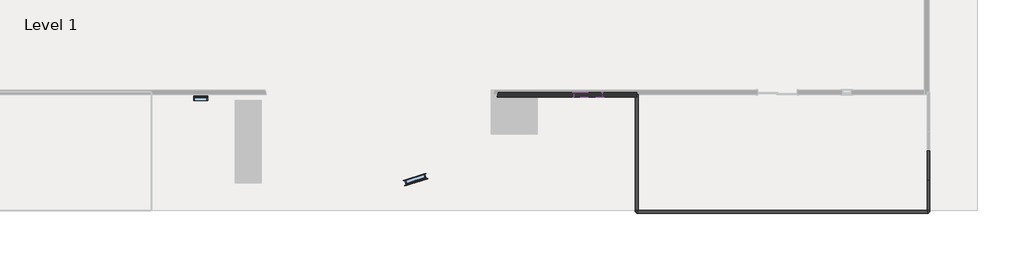
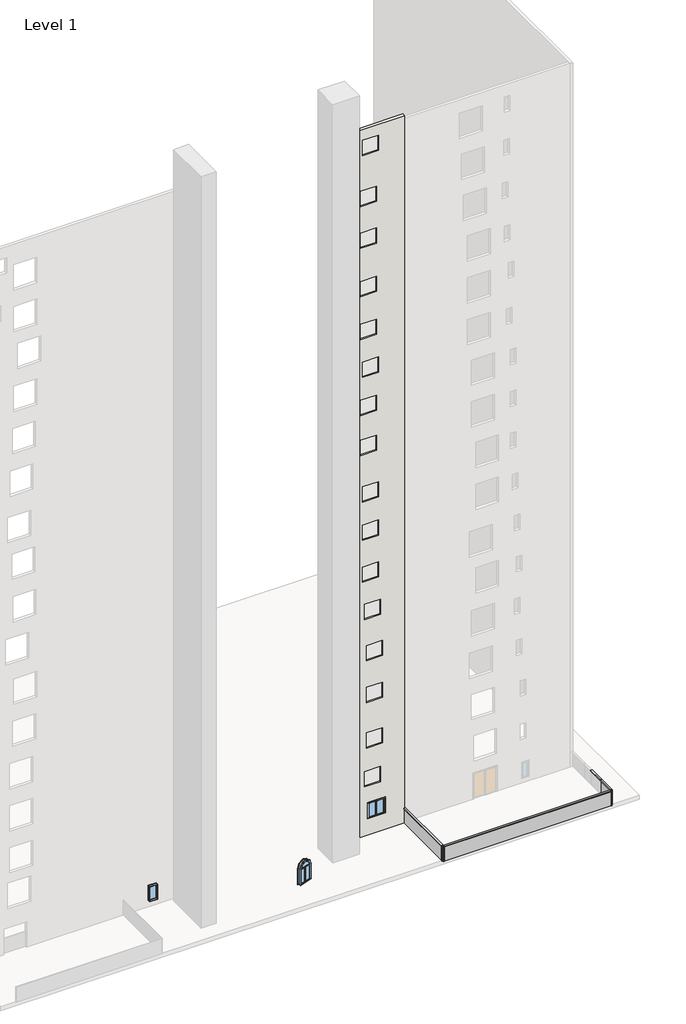
# One storey, part 2 of 3: 8 members, 3 plates, 3 windows, 1 wall.
"""IFC4 building model written with IfcOpenShell, lengths in millimetres."""

from ifc_helpers import new_model, si_unit, frame, origin, place, context, project, spatial, polyline, circle_curve, transform, mapped, element, save
from ifc_brep_helpers import plane_surface, revolved_surface, advanced_brep
from components import member_75074519, member_7da84c5f, member_82acb0db, member_acf158a7, member_d37749d9, system_panel_glazed_a0600ee7, system_panel_glazed_16aad0d4, system_panel_glazed_fdf8efc7, window_cf4adaea, window_0862ab64, window_80bd9af0

model = new_model("IFC4")

# Units and contexts
model_context = context("Model", 3, world=origin())
ifc_project = project(units=[si_unit("LENGTHUNIT", "METRE", prefix="MILLI")], contexts=[model_context])

# Site, building, storey
site = spatial("IfcSite", under=ifc_project)
building = spatial("IfcBuilding", under=site)
storey = spatial("IfcBuildingStorey", under=building, Name="Level 1", Elevation=0.0)

# Members
placement = place(None, origin())
member_shape = member_75074519(model_context)
element("IfcMember", 1, ObjectType="Rectangular Mullion : 2.5\" x 5\" rectangular", at=placement, inside=storey, context=model_context, shape_type="MappedRepresentation", body=[
    mapped(member_shape, transform((12667.5594464, -17598.421855, 1219.2), x_axis=(0.0, -1.0, 0.0), y_axis=(1.0, 0.0, 0.0), z_axis=(0.0, 0.0, 1.0))),
])
element("IfcMember", 2, ObjectType="Rectangular Mullion : 2.5\" x 5\" rectangular", at=placement, inside=storey, context=model_context, shape_type="MappedRepresentation", body=[
    mapped(member_shape, transform((25464.414721, -17598.421855, 1219.2), x_axis=(1.0, 0.0, 0.0), y_axis=(0.0, 1.0, 0.0), z_axis=(0.0, 0.0, 1.0))),
])
element("IfcMember", 3, ObjectType="Rectangular Mullion : 2.5\" x 5\" rectangular", at=placement, inside=storey, context=model_context, shape_type="MappedRepresentation", body=[
    mapped(member_shape, transform((12667.5594464, -17598.421855, 0.0), x_axis=(-1.0, 0.0, 0.0), y_axis=(0.0, 1.0, 0.0), z_axis=(0.0, 0.0, -1.0))),
])
element("IfcMember", 4, ObjectType="Rectangular Mullion : 2.5\" x 5\" rectangular", at=placement, inside=storey, context=model_context, shape_type="MappedRepresentation", body=[
    mapped(member_shape, transform((25464.414721, -17598.421855, 0.0), x_axis=(0.0, -1.0, 0.0), y_axis=(-1.0, 0.0, 0.0), z_axis=(0.0, 0.0, -1.0))),
])
member_2_shape = member_7da84c5f(model_context)
element("IfcMember", 5, ObjectType="Rectangular Mullion : 2.5\" x 5\" rectangular", at=placement, inside=storey, context=model_context, shape_type="MappedRepresentation", body=[
    mapped(member_2_shape, transform((12667.5594464, -12456.3237084, 1219.2), x_axis=(0.0, 0.0, 1.0), y_axis=(1.0, 0.0, 0.0), z_axis=(0.0, 1.0, 0.0))),
])
member_3_shape = member_82acb0db(model_context)
element("IfcMember", 6, ObjectType="Rectangular Mullion : 2.5\" x 5\" rectangular", at=placement, inside=storey, context=model_context, shape_type="MappedRepresentation", body=[
    mapped(member_3_shape, transform((12731.0594464, -17598.421855, 1219.2), x_axis=(0.0, 0.0, 1.0), y_axis=(0.0, 1.0, 0.0), z_axis=(-1.0, 0.0, 0.0))),
])
member_4_shape = member_acf158a7(model_context)
element("IfcMember", 7, ObjectType="Rectangular Mullion : 2.5\" x 5\" rectangular", at=placement, inside=storey, context=model_context, shape_type="MappedRepresentation", body=[
    mapped(member_4_shape, transform((25464.414721, -16226.821855, 1219.2), x_axis=(0.0, 0.0, 1.0), y_axis=(-1.0, 0.0, 0.0), z_axis=(0.0, -1.0, 0.0))),
])
member_5_shape = member_d37749d9(model_context)
element("IfcMember", 8, ObjectType="Rectangular Mullion : 2.5\" x 5\" rectangular", at=placement, inside=storey, context=model_context, shape_type="MappedRepresentation", body=[
    mapped(member_5_shape, transform((25464.414721, -17534.921855, 1219.2), x_axis=(0.0, 0.0, 1.0), y_axis=(-1.0, 0.0, 0.0), z_axis=(0.0, -1.0, 0.0))),
])

# Plates
system_panel_glazed_shape = system_panel_glazed_a0600ee7(model_context)
element("IfcPlate", 9, ObjectType="System Panel : Glazed", at=placement, inside=storey, context=model_context, shape_type="MappedRepresentation", body=[
    mapped(system_panel_glazed_shape, transform((12667.5594464, -14995.6227817, 0.0), x_axis=(0.0, 1.0, 0.0), y_axis=(-1.0, 0.0, 0.0), z_axis=(0.0, 0.0, 1.0))),
])
system_panel_glazed_2_shape = system_panel_glazed_16aad0d4(model_context)
element("IfcPlate", 10, ObjectType="System Panel : Glazed", at=placement, inside=storey, context=model_context, shape_type="MappedRepresentation", body=[
    mapped(system_panel_glazed_2_shape, transform((19065.9870837, -17598.421855, 0.0), x_axis=(-1.0, 0.0, 0.0), y_axis=(0.0, -1.0, 0.0), z_axis=(0.0, 0.0, 1.0))),
])
system_panel_glazed_3_shape = system_panel_glazed_fdf8efc7(model_context)
element("IfcPlate", 11, ObjectType="System Panel : Glazed", at=placement, inside=storey, context=model_context, shape_type="MappedRepresentation", body=[
    mapped(system_panel_glazed_3_shape, transform((25464.414721, -16880.871855, 0.0), x_axis=(0.0, -1.0, 0.0), y_axis=(1.0, 0.0, 0.0), z_axis=(0.0, 0.0, 1.0))),
])

# Wall
element("IfcWall", 12, ObjectType="Generic - 8\"", at=placement, inside=storey, context=model_context, shape_type="AdvancedBrep", body=[
    advanced_brep(
    [(6546.3952465, -12557.9237084, 56730.1367162), (6546.3952465, -12557.9237084, 0.0), (12667.5594464, -12557.9237084, 0.0), (12667.5594464, -12557.9237084, 56730.1367162), (9467.1594464, -12557.9237084, 55849.139368), (10686.3594464, -12557.9237084, 55849.139368), (10686.3594464, -12557.9237084, 54629.939368), (9467.1594464, -12557.9237084, 54629.939368), (9314.7594464, -12557.9237084, 51816.0), (10533.9594464, -12557.9237084, 51816.0), (10533.9594464, -12557.9237084, 50596.8), (9314.7594464, -12557.9237084, 50596.8), (9314.7594464, -12557.9237084, 48463.2), (10533.9594464, -12557.9237084, 48463.2), (10533.9594464, -12557.9237084, 47244.0), (9314.7594464, -12557.9237084, 47244.0), (9314.7594464, -12557.9237084, 44593.7672913), (10533.9594464, -12557.9237084, 44593.7672913), (10533.9594464, -12557.9237084, 43374.5672913), (9314.7594464, -12557.9237084, 43374.5672913), (9314.7594464, -12557.9237084, 41155.7053459), (10533.9594464, -12557.9237084, 41155.7053459), (10533.9594464, -12557.9237084, 39936.5053459), (9314.7594464, -12557.9237084, 39936.5053459), (9467.1594464, -12557.9237084, 38064.0788406), (10686.3594464, -12557.9237084, 38064.0788406), (10686.3594464, -12557.9237084, 36844.8788406), (9467.1594464, -12557.9237084, 36844.8788406), (9314.7594464, -12557.9237084, 35052.0), (10533.9594464, -12557.9237084, 35052.0), (10533.9594464, -12557.9237084, 33832.8), (9314.7594464, -12557.9237084, 33832.8), (9314.7594464, -12557.9237084, 31851.4859618), (10533.9594464, -12557.9237084, 31851.4859618), (10533.9594464, -12557.9237084, 30632.2859618), (9314.7594464, -12557.9237084, 30632.2859618), (9467.1594464, -12557.9237084, 28064.0725002), (10686.3594464, -12557.9237084, 28064.0725002), (10686.3594464, -12557.9237084, 26844.8725002), (9467.1594464, -12557.9237084, 26844.8725002), (9467.1594464, -12557.9237084, 24993.6), (10686.3594464, -12557.9237084, 24993.6), (10686.3594464, -12557.9237084, 23774.4), (9467.1594464, -12557.9237084, 23774.4), (9467.1594464, -12557.9237084, 21640.8), (10686.3594464, -12557.9237084, 21640.8), (10686.3594464, -12557.9237084, 20421.6), (9467.1594464, -12557.9237084, 20421.6), (9619.5594464, -12557.9237084, 18592.8), (10838.7594464, -12557.9237084, 18592.8), (10838.7594464, -12557.9237084, 17373.6), (9619.5594464, -12557.9237084, 17373.6), (9771.9594464, -12557.9237084, 15240.0), (10991.1594464, -12557.9237084, 15240.0), (10991.1594464, -12557.9237084, 14020.8), (9771.9594464, -12557.9237084, 14020.8), (9771.9594464, -12557.9237084, 11887.2), (10991.1594464, -12557.9237084, 11887.2), (10991.1594464, -12557.9237084, 10668.0), (9771.9594464, -12557.9237084, 10668.0), (9771.9594464, -12557.9237084, 8229.6), (10991.1594464, -12557.9237084, 8229.6), (10991.1594464, -12557.9237084, 7010.4), (9771.9594464, -12557.9237084, 7010.4), (9619.5594464, -12557.9237084, 5181.6), (10838.7594464, -12557.9237084, 5181.6), (10838.7594464, -12557.9237084, 3962.4), (9619.5594464, -12557.9237084, 3962.4), (9924.3594464, -12557.9237084, 2560.5553326), (11143.5594464, -12557.9237084, 2560.5553326), (11143.5594464, -12557.9237084, 1341.3553326), (9924.3594464, -12557.9237084, 1341.3553326), (6594.6209909, -12354.7237084, 0.0), (6594.6209909, -12354.7237084, 56425.3367162), (6594.6209909, -12354.7237084, 56730.1367162), (12667.5594464, -12354.7237084, 56730.1367162), (12667.5594464, -12354.7237084, 0.0), (9467.1594464, -12354.7237084, 55849.139368), (9467.1594464, -12354.7237084, 54629.939368), (10686.3594464, -12354.7237084, 54629.939368), (10686.3594464, -12354.7237084, 55849.139368), (9314.7594464, -12354.7237084, 51816.0), (9314.7594464, -12354.7237084, 50596.8), (10533.9594464, -12354.7237084, 50596.8), (10533.9594464, -12354.7237084, 51816.0), (9314.7594464, -12354.7237084, 48463.2), (9314.7594464, -12354.7237084, 47244.0), (10533.9594464, -12354.7237084, 47244.0), (10533.9594464, -12354.7237084, 48463.2), (9314.7594464, -12354.7237084, 44593.7672913), (9314.7594464, -12354.7237084, 43374.5672913), (10533.9594464, -12354.7237084, 43374.5672913), (10533.9594464, -12354.7237084, 44593.7672913), (9314.7594464, -12354.7237084, 41155.7053459), (9314.7594464, -12354.7237084, 39936.5053459), (10533.9594464, -12354.7237084, 39936.5053459), (10533.9594464, -12354.7237084, 41155.7053459), (9467.1594464, -12354.7237084, 38064.0788406), (9467.1594464, -12354.7237084, 36844.8788406), (10686.3594464, -12354.7237084, 36844.8788406), (10686.3594464, -12354.7237084, 38064.0788406), (9314.7594464, -12354.7237084, 35052.0), (9314.7594464, -12354.7237084, 33832.8), (10533.9594464, -12354.7237084, 33832.8), (10533.9594464, -12354.7237084, 35052.0), (9314.7594464, -12354.7237084, 31851.4859618), (9314.7594464, -12354.7237084, 30632.2859618), (10533.9594464, -12354.7237084, 30632.2859618), (10533.9594464, -12354.7237084, 31851.4859618), (9467.1594464, -12354.7237084, 28064.0725002), (9467.1594464, -12354.7237084, 26844.8725002), (10686.3594464, -12354.7237084, 26844.8725002), (10686.3594464, -12354.7237084, 28064.0725002), (9467.1594464, -12354.7237084, 24993.6), (9467.1594464, -12354.7237084, 23774.4), (10686.3594464, -12354.7237084, 23774.4), (10686.3594464, -12354.7237084, 24993.6), (9467.1594464, -12354.7237084, 21640.8), (9467.1594464, -12354.7237084, 20421.6), (10686.3594464, -12354.7237084, 20421.6), (10686.3594464, -12354.7237084, 21640.8), (9619.5594464, -12354.7237084, 18592.8), (9619.5594464, -12354.7237084, 17373.6), (10838.7594464, -12354.7237084, 17373.6), (10838.7594464, -12354.7237084, 18592.8), (9771.9594464, -12354.7237084, 15240.0), (9771.9594464, -12354.7237084, 14020.8), (10991.1594464, -12354.7237084, 14020.8), (10991.1594464, -12354.7237084, 15240.0), (9771.9594464, -12354.7237084, 11887.2), (9771.9594464, -12354.7237084, 10668.0), (10991.1594464, -12354.7237084, 10668.0), (10991.1594464, -12354.7237084, 11887.2), (9771.9594464, -12354.7237084, 8229.6), (9771.9594464, -12354.7237084, 7010.4), (10991.1594464, -12354.7237084, 7010.4), (10991.1594464, -12354.7237084, 8229.6), (9619.5594464, -12354.7237084, 5181.6), (9619.5594464, -12354.7237084, 3962.4), (10838.7594464, -12354.7237084, 3962.4), (10838.7594464, -12354.7237084, 5181.6), (9924.3594464, -12354.7237084, 2560.5553326), (9924.3594464, -12354.7237084, 1341.3553326), (11143.5594464, -12354.7237084, 1341.3553326), (11143.5594464, -12354.7237084, 2560.5553326), (6571.5594428, -12456.3237235, 0.0)],
    [
        (0, 1),
        (1, 2),
        (2, 3),
        (3, 0),
        (4, 5),
        (5, 6),
        (6, 7),
        (7, 4),
        (8, 9),
        (9, 10),
        (10, 11),
        (11, 8),
        (12, 13),
        (13, 14),
        (14, 15),
        (15, 12),
        (16, 17),
        (17, 18),
        (18, 19),
        (19, 16),
        (20, 21),
        (21, 22),
        (22, 23),
        (23, 20),
        (24, 25),
        (25, 26),
        (26, 27),
        (27, 24),
        (28, 29),
        (29, 30),
        (30, 31),
        (31, 28),
        (32, 33),
        (33, 34),
        (34, 35),
        (35, 32),
        (36, 37),
        (37, 38),
        (38, 39),
        (39, 36),
        (40, 41),
        (41, 42),
        (42, 43),
        (43, 40),
        (44, 45),
        (45, 46),
        (46, 47),
        (47, 44),
        (48, 49),
        (49, 50),
        (50, 51),
        (51, 48),
        (52, 53),
        (53, 54),
        (54, 55),
        (55, 52),
        (56, 57),
        (57, 58),
        (58, 59),
        (59, 56),
        (60, 61),
        (61, 62),
        (62, 63),
        (63, 60),
        (64, 65),
        (65, 66),
        (66, 67),
        (67, 64),
        (68, 69),
        (69, 70),
        (70, 71),
        (71, 68),
        (72, 73),
        (73, 74),
        (74, 75),
        (75, 76),
        (76, 72),
        (77, 78),
        (78, 79),
        (79, 80),
        (80, 77),
        (81, 82),
        (82, 83),
        (83, 84),
        (84, 81),
        (85, 86),
        (86, 87),
        (87, 88),
        (88, 85),
        (89, 90),
        (90, 91),
        (91, 92),
        (92, 89),
        (93, 94),
        (94, 95),
        (95, 96),
        (96, 93),
        (97, 98),
        (98, 99),
        (99, 100),
        (100, 97),
        (101, 102),
        (102, 103),
        (103, 104),
        (104, 101),
        (105, 106),
        (106, 107),
        (107, 108),
        (108, 105),
        (109, 110),
        (110, 111),
        (111, 112),
        (112, 109),
        (113, 114),
        (114, 115),
        (115, 116),
        (116, 113),
        (117, 118),
        (118, 119),
        (119, 120),
        (120, 117),
        (121, 122),
        (122, 123),
        (123, 124),
        (124, 121),
        (125, 126),
        (126, 127),
        (127, 128),
        (128, 125),
        (129, 130),
        (130, 131),
        (131, 132),
        (132, 129),
        (133, 134),
        (134, 135),
        (135, 136),
        (136, 133),
        (137, 138),
        (138, 139),
        (139, 140),
        (140, 137),
        (141, 142),
        (142, 143),
        (143, 144),
        (144, 141),
        (1, 145, circle_curve(frame((1385.214721, -11225.6906671, 0.0), z_axis=(0.0, 0.0, 1.0), x_axis=(1.0, 0.0, 0.0)), 5330.3498284)),
        (145, 72, circle_curve(frame((1385.214721, -11225.6906671, 0.0), z_axis=(0.0, 0.0, 1.0), x_axis=(1.0, 0.0, 0.0)), 5330.3498284)),
        (76, 2),
        (75, 3),
        (74, 0, circle_curve(frame((1385.214721, -11225.6906671, 56730.1367162), z_axis=(0.0, 0.0, -1.0), x_axis=(1.0, 0.0, 0.0)), 5330.3498284)),
        (77, 4),
        (7, 78),
        (6, 79),
        (5, 80),
        (81, 8),
        (11, 82),
        (10, 83),
        (9, 84),
        (85, 12),
        (15, 86),
        (14, 87),
        (13, 88),
        (89, 16),
        (19, 90),
        (18, 91),
        (17, 92),
        (93, 20),
        (23, 94),
        (22, 95),
        (21, 96),
        (97, 24),
        (27, 98),
        (26, 99),
        (25, 100),
        (101, 28),
        (31, 102),
        (30, 103),
        (29, 104),
        (105, 32),
        (35, 106),
        (34, 107),
        (33, 108),
        (109, 36),
        (39, 110),
        (38, 111),
        (37, 112),
        (113, 40),
        (43, 114),
        (42, 115),
        (41, 116),
        (117, 44),
        (47, 118),
        (46, 119),
        (45, 120),
        (121, 48),
        (51, 122),
        (50, 123),
        (49, 124),
        (125, 52),
        (55, 126),
        (54, 127),
        (53, 128),
        (129, 56),
        (59, 130),
        (58, 131),
        (57, 132),
        (133, 60),
        (63, 134),
        (62, 135),
        (61, 136),
        (137, 64),
        (67, 138),
        (66, 139),
        (65, 140),
        (141, 68),
        (71, 142),
        (70, 143),
        (69, 144),
    ],
    [
        plane_surface(frame((6571.5594464, -12557.9237084, 0.0), z_axis=(0.0, -1.0, 0.0), x_axis=(1.0, 0.0, 0.0))),
        plane_surface(frame((6571.5594464, -12354.7237084, 0.0), z_axis=(0.0, 1.0, 0.0), x_axis=(-1.0, 0.0, 0.0))),
        plane_surface(frame((6467.0812172, -12557.9237084, 0.0), z_axis=(0.0, 0.0, -1.0), x_axis=(0.0, 1.0, 0.0))),
        plane_surface(frame((12667.5594464, -12557.9237084, 0.0), z_axis=(1.0, 0.0, 0.0), x_axis=(0.0, 1.0, 0.0))),
        plane_surface(frame((12667.5594464, -12557.9237084, 56730.1367162), z_axis=(0.0, 0.0, 1.0), x_axis=(0.0, 1.0, 0.0))),
        revolved_surface(polyline([(6715.5645494, -11225.6906671, 56730.1367162), (6715.5645494, -11225.6906671, 0.0)]), (1385.214721, -11225.6906671, 0.0), (0.0, 0.0, 1.0)),
        plane_surface(frame((9467.1594464, -12354.7237084, 55849.139368), z_axis=(1.0, 0.0, 0.0), x_axis=(0.0, -1.0, 0.0))),
        plane_surface(frame((9467.1594464, -12354.7237084, 54629.939368), z_axis=(0.0, 0.0, 1.0), x_axis=(0.0, -1.0, 0.0))),
        plane_surface(frame((10686.3594464, -12354.7237084, 54629.939368), z_axis=(-1.0, 0.0, 0.0), x_axis=(0.0, -1.0, 0.0))),
        plane_surface(frame((10686.3594464, -12354.7237084, 55849.139368), z_axis=(0.0, 0.0, -1.0), x_axis=(0.0, -1.0, 0.0))),
        plane_surface(frame((9314.7594464, -12354.7237084, 51816.0), z_axis=(1.0, 0.0, 0.0), x_axis=(0.0, -1.0, 0.0))),
        plane_surface(frame((9314.7594464, -12354.7237084, 50596.8), z_axis=(0.0, 0.0, 1.0), x_axis=(0.0, -1.0, 0.0))),
        plane_surface(frame((10533.9594464, -12354.7237084, 50596.8), z_axis=(-1.0, 0.0, 0.0), x_axis=(0.0, -1.0, 0.0))),
        plane_surface(frame((10533.9594464, -12354.7237084, 51816.0), z_axis=(0.0, 0.0, -1.0), x_axis=(0.0, -1.0, 0.0))),
        plane_surface(frame((9314.7594464, -12354.7237084, 48463.2), z_axis=(1.0, 0.0, 0.0), x_axis=(0.0, -1.0, 0.0))),
        plane_surface(frame((9314.7594464, -12354.7237084, 47244.0), z_axis=(0.0, 0.0, 1.0), x_axis=(0.0, -1.0, 0.0))),
        plane_surface(frame((10533.9594464, -12354.7237084, 47244.0), z_axis=(-1.0, 0.0, 0.0), x_axis=(0.0, -1.0, 0.0))),
        plane_surface(frame((10533.9594464, -12354.7237084, 48463.2), z_axis=(0.0, 0.0, -1.0), x_axis=(0.0, -1.0, 0.0))),
        plane_surface(frame((9314.7594464, -12354.7237084, 44593.7672913), z_axis=(1.0, 0.0, 0.0), x_axis=(0.0, -1.0, 0.0))),
        plane_surface(frame((9314.7594464, -12354.7237084, 43374.5672913), z_axis=(0.0, 0.0, 1.0), x_axis=(0.0, -1.0, 0.0))),
        plane_surface(frame((10533.9594464, -12354.7237084, 43374.5672913), z_axis=(-1.0, 0.0, 0.0), x_axis=(0.0, -1.0, 0.0))),
        plane_surface(frame((10533.9594464, -12354.7237084, 44593.7672913), z_axis=(0.0, 0.0, -1.0), x_axis=(0.0, -1.0, 0.0))),
        plane_surface(frame((9314.7594464, -12354.7237084, 41155.7053459), z_axis=(1.0, 0.0, 0.0), x_axis=(0.0, -1.0, 0.0))),
        plane_surface(frame((9314.7594464, -12354.7237084, 39936.5053459), z_axis=(0.0, 0.0, 1.0), x_axis=(0.0, -1.0, 0.0))),
        plane_surface(frame((10533.9594464, -12354.7237084, 39936.5053459), z_axis=(-1.0, 0.0, 0.0), x_axis=(0.0, -1.0, 0.0))),
        plane_surface(frame((10533.9594464, -12354.7237084, 41155.7053459), z_axis=(0.0, 0.0, -1.0), x_axis=(0.0, -1.0, 0.0))),
        plane_surface(frame((9467.1594464, -12354.7237084, 38064.0788406), z_axis=(1.0, 0.0, 0.0), x_axis=(0.0, -1.0, 0.0))),
        plane_surface(frame((9467.1594464, -12354.7237084, 36844.8788406), z_axis=(0.0, 0.0, 1.0), x_axis=(0.0, -1.0, 0.0))),
        plane_surface(frame((10686.3594464, -12354.7237084, 36844.8788406), z_axis=(-1.0, 0.0, 0.0), x_axis=(0.0, -1.0, 0.0))),
        plane_surface(frame((10686.3594464, -12354.7237084, 38064.0788406), z_axis=(0.0, 0.0, -1.0), x_axis=(0.0, -1.0, 0.0))),
        plane_surface(frame((9314.7594464, -12354.7237084, 35052.0), z_axis=(1.0, 0.0, 0.0), x_axis=(0.0, -1.0, 0.0))),
        plane_surface(frame((9314.7594464, -12354.7237084, 33832.8), z_axis=(0.0, 0.0, 1.0), x_axis=(0.0, -1.0, 0.0))),
        plane_surface(frame((10533.9594464, -12354.7237084, 33832.8), z_axis=(-1.0, 0.0, 0.0), x_axis=(0.0, -1.0, 0.0))),
        plane_surface(frame((10533.9594464, -12354.7237084, 35052.0), z_axis=(0.0, 0.0, -1.0), x_axis=(0.0, -1.0, 0.0))),
        plane_surface(frame((9314.7594464, -12354.7237084, 31851.4859618), z_axis=(1.0, 0.0, 0.0), x_axis=(0.0, -1.0, 0.0))),
        plane_surface(frame((9314.7594464, -12354.7237084, 30632.2859618), z_axis=(0.0, 0.0, 1.0), x_axis=(0.0, -1.0, 0.0))),
        plane_surface(frame((10533.9594464, -12354.7237084, 30632.2859618), z_axis=(-1.0, 0.0, 0.0), x_axis=(0.0, -1.0, 0.0))),
        plane_surface(frame((10533.9594464, -12354.7237084, 31851.4859618), z_axis=(0.0, 0.0, -1.0), x_axis=(0.0, -1.0, 0.0))),
        plane_surface(frame((9467.1594464, -12354.7237084, 28064.0725002), z_axis=(1.0, 0.0, 0.0), x_axis=(0.0, -1.0, 0.0))),
        plane_surface(frame((9467.1594464, -12354.7237084, 26844.8725002), z_axis=(0.0, 0.0, 1.0), x_axis=(0.0, -1.0, 0.0))),
        plane_surface(frame((10686.3594464, -12354.7237084, 26844.8725002), z_axis=(-1.0, 0.0, 0.0), x_axis=(0.0, -1.0, 0.0))),
        plane_surface(frame((10686.3594464, -12354.7237084, 28064.0725002), z_axis=(0.0, 0.0, -1.0), x_axis=(0.0, -1.0, 0.0))),
        plane_surface(frame((9467.1594464, -12354.7237084, 24993.6), z_axis=(1.0, 0.0, 0.0), x_axis=(0.0, -1.0, 0.0))),
        plane_surface(frame((9467.1594464, -12354.7237084, 23774.4), z_axis=(0.0, 0.0, 1.0), x_axis=(0.0, -1.0, 0.0))),
        plane_surface(frame((10686.3594464, -12354.7237084, 23774.4), z_axis=(-1.0, 0.0, 0.0), x_axis=(0.0, -1.0, 0.0))),
        plane_surface(frame((10686.3594464, -12354.7237084, 24993.6), z_axis=(0.0, 0.0, -1.0), x_axis=(0.0, -1.0, 0.0))),
        plane_surface(frame((9467.1594464, -12354.7237084, 21640.8), z_axis=(1.0, 0.0, 0.0), x_axis=(0.0, -1.0, 0.0))),
        plane_surface(frame((9467.1594464, -12354.7237084, 20421.6), z_axis=(0.0, 0.0, 1.0), x_axis=(0.0, -1.0, 0.0))),
        plane_surface(frame((10686.3594464, -12354.7237084, 20421.6), z_axis=(-1.0, 0.0, 0.0), x_axis=(0.0, -1.0, 0.0))),
        plane_surface(frame((10686.3594464, -12354.7237084, 21640.8), z_axis=(0.0, 0.0, -1.0), x_axis=(0.0, -1.0, 0.0))),
        plane_surface(frame((9619.5594464, -12354.7237084, 18592.8), z_axis=(1.0, 0.0, 0.0), x_axis=(0.0, -1.0, 0.0))),
        plane_surface(frame((9619.5594464, -12354.7237084, 17373.6), z_axis=(0.0, 0.0, 1.0), x_axis=(0.0, -1.0, 0.0))),
        plane_surface(frame((10838.7594464, -12354.7237084, 17373.6), z_axis=(-1.0, 0.0, 0.0), x_axis=(0.0, -1.0, 0.0))),
        plane_surface(frame((10838.7594464, -12354.7237084, 18592.8), z_axis=(0.0, 0.0, -1.0), x_axis=(0.0, -1.0, 0.0))),
        plane_surface(frame((9771.9594464, -12354.7237084, 15240.0), z_axis=(1.0, 0.0, 0.0), x_axis=(0.0, -1.0, 0.0))),
        plane_surface(frame((9771.9594464, -12354.7237084, 14020.8), z_axis=(0.0, 0.0, 1.0), x_axis=(0.0, -1.0, 0.0))),
        plane_surface(frame((10991.1594464, -12354.7237084, 14020.8), z_axis=(-1.0, 0.0, 0.0), x_axis=(0.0, -1.0, 0.0))),
        plane_surface(frame((10991.1594464, -12354.7237084, 15240.0), z_axis=(0.0, 0.0, -1.0), x_axis=(0.0, -1.0, 0.0))),
        plane_surface(frame((9771.9594464, -12354.7237084, 11887.2), z_axis=(1.0, 0.0, 0.0), x_axis=(0.0, -1.0, 0.0))),
        plane_surface(frame((9771.9594464, -12354.7237084, 10668.0), z_axis=(0.0, 0.0, 1.0), x_axis=(0.0, -1.0, 0.0))),
        plane_surface(frame((10991.1594464, -12354.7237084, 10668.0), z_axis=(-1.0, 0.0, 0.0), x_axis=(0.0, -1.0, 0.0))),
        plane_surface(frame((10991.1594464, -12354.7237084, 11887.2), z_axis=(0.0, 0.0, -1.0), x_axis=(0.0, -1.0, 0.0))),
        plane_surface(frame((9771.9594464, -12354.7237084, 8229.6), z_axis=(1.0, 0.0, 0.0), x_axis=(0.0, -1.0, 0.0))),
        plane_surface(frame((9771.9594464, -12354.7237084, 7010.4), z_axis=(0.0, 0.0, 1.0), x_axis=(0.0, -1.0, 0.0))),
        plane_surface(frame((10991.1594464, -12354.7237084, 7010.4), z_axis=(-1.0, 0.0, 0.0), x_axis=(0.0, -1.0, 0.0))),
        plane_surface(frame((10991.1594464, -12354.7237084, 8229.6), z_axis=(0.0, 0.0, -1.0), x_axis=(0.0, -1.0, 0.0))),
        plane_surface(frame((9619.5594464, -12354.7237084, 5181.6), z_axis=(1.0, 0.0, 0.0), x_axis=(0.0, -1.0, 0.0))),
        plane_surface(frame((9619.5594464, -12354.7237084, 3962.4), z_axis=(0.0, 0.0, 1.0), x_axis=(0.0, -1.0, 0.0))),
        plane_surface(frame((10838.7594464, -12354.7237084, 3962.4), z_axis=(-1.0, 0.0, 0.0), x_axis=(0.0, -1.0, 0.0))),
        plane_surface(frame((10838.7594464, -12354.7237084, 5181.6), z_axis=(0.0, 0.0, -1.0), x_axis=(0.0, -1.0, 0.0))),
        plane_surface(frame((9924.3594464, -12354.7237084, 2560.5553326), z_axis=(1.0, 0.0, 0.0), x_axis=(0.0, -1.0, 0.0))),
        plane_surface(frame((9924.3594464, -12354.7237084, 1341.3553326), z_axis=(0.0, 0.0, 1.0), x_axis=(0.0, -1.0, 0.0))),
        plane_surface(frame((11143.5594464, -12354.7237084, 1341.3553326), z_axis=(-1.0, 0.0, 0.0), x_axis=(0.0, -1.0, 0.0))),
        plane_surface(frame((11143.5594464, -12354.7237084, 2560.5553326), z_axis=(0.0, 0.0, -1.0), x_axis=(0.0, -1.0, 0.0))),
    ],
    [
        (0, [[1, 2, 3, 4], [5, 6, 7, 8], [9, 10, 11, 12], [13, 14, 15, 16], [17, 18, 19, 20], [21, 22, 23, 24], [25, 26, 27, 28], [29, 30, 31, 32], [33, 34, 35, 36], [37, 38, 39, 40], [41, 42, 43, 44], [45, 46, 47, 48], [49, 50, 51, 52], [53, 54, 55, 56], [57, 58, 59, 60], [61, 62, 63, 64], [65, 66, 67, 68], [69, 70, 71, 72]]),
        (1, [[73, 74, 75, 76, 77], [78, 79, 80, 81], [82, 83, 84, 85], [86, 87, 88, 89], [90, 91, 92, 93], [94, 95, 96, 97], [98, 99, 100, 101], [102, 103, 104, 105], [106, 107, 108, 109], [110, 111, 112, 113], [114, 115, 116, 117], [118, 119, 120, 121], [122, 123, 124, 125], [126, 127, 128, 129], [130, 131, 132, 133], [134, 135, 136, 137], [138, 139, 140, 141], [142, 143, 144, 145]]),
        (2, [[-2, 146, 147, -77, 148]]),
        (3, [[-3, -148, -76, 149]]),
        (4, [[-4, -149, -75, 150]]),
        (5, [[-150, -74, -73, -147, -146, -1]]),
        (6, [[-78, 151, -8, 152]]),
        (7, [[-79, -152, -7, 153]]),
        (8, [[-80, -153, -6, 154]]),
        (9, [[-81, -154, -5, -151]]),
        (10, [[-82, 155, -12, 156]]),
        (11, [[-83, -156, -11, 157]]),
        (12, [[-84, -157, -10, 158]]),
        (13, [[-85, -158, -9, -155]]),
        (14, [[-86, 159, -16, 160]]),
        (15, [[-87, -160, -15, 161]]),
        (16, [[-88, -161, -14, 162]]),
        (17, [[-89, -162, -13, -159]]),
        (18, [[-90, 163, -20, 164]]),
        (19, [[-91, -164, -19, 165]]),
        (20, [[-92, -165, -18, 166]]),
        (21, [[-93, -166, -17, -163]]),
        (22, [[-94, 167, -24, 168]]),
        (23, [[-95, -168, -23, 169]]),
        (24, [[-96, -169, -22, 170]]),
        (25, [[-97, -170, -21, -167]]),
        (26, [[-98, 171, -28, 172]]),
        (27, [[-99, -172, -27, 173]]),
        (28, [[-100, -173, -26, 174]]),
        (29, [[-101, -174, -25, -171]]),
        (30, [[-102, 175, -32, 176]]),
        (31, [[-103, -176, -31, 177]]),
        (32, [[-104, -177, -30, 178]]),
        (33, [[-105, -178, -29, -175]]),
        (34, [[-106, 179, -36, 180]]),
        (35, [[-107, -180, -35, 181]]),
        (36, [[-108, -181, -34, 182]]),
        (37, [[-109, -182, -33, -179]]),
        (38, [[-110, 183, -40, 184]]),
        (39, [[-111, -184, -39, 185]]),
        (40, [[-112, -185, -38, 186]]),
        (41, [[-113, -186, -37, -183]]),
        (42, [[-114, 187, -44, 188]]),
        (43, [[-115, -188, -43, 189]]),
        (44, [[-116, -189, -42, 190]]),
        (45, [[-117, -190, -41, -187]]),
        (46, [[-118, 191, -48, 192]]),
        (47, [[-119, -192, -47, 193]]),
        (48, [[-120, -193, -46, 194]]),
        (49, [[-121, -194, -45, -191]]),
        (50, [[-122, 195, -52, 196]]),
        (51, [[-123, -196, -51, 197]]),
        (52, [[-124, -197, -50, 198]]),
        (53, [[-125, -198, -49, -195]]),
        (54, [[-126, 199, -56, 200]]),
        (55, [[-127, -200, -55, 201]]),
        (56, [[-128, -201, -54, 202]]),
        (57, [[-129, -202, -53, -199]]),
        (58, [[-130, 203, -60, 204]]),
        (59, [[-131, -204, -59, 205]]),
        (60, [[-132, -205, -58, 206]]),
        (61, [[-133, -206, -57, -203]]),
        (62, [[-134, 207, -64, 208]]),
        (63, [[-135, -208, -63, 209]]),
        (64, [[-136, -209, -62, 210]]),
        (65, [[-137, -210, -61, -207]]),
        (66, [[-138, 211, -68, 212]]),
        (67, [[-139, -212, -67, 213]]),
        (68, [[-140, -213, -66, 214]]),
        (69, [[-141, -214, -65, -211]]),
        (70, [[-142, 215, -72, 216]]),
        (71, [[-143, -216, -71, 217]]),
        (72, [[-144, -217, -70, 218]]),
        (73, [[-145, -218, -69, -215]]),
    ],
),
])

# Windows
window_shape = window_cf4adaea(model_context)
element("IfcWindow", 13, ObjectType="36\" x 48\"", at=placement, inside=storey, context=model_context, shape_type="MappedRepresentation", body=[
    mapped(window_shape, transform((2966.4751004, -16189.0024864, 0.0), x_axis=(-0.9532786010374131, -0.3020925500639706, 0.0), y_axis=(0.3020925500639706, -0.9532786010374131, 0.0), z_axis=(0.0, 0.0, 1.0))),
])
window_2_shape = window_0862ab64(model_context)
element("IfcWindow", 14, ObjectType="Casement Dbl with Trim : 48\" x 48\"", at=placement, inside=storey, context=model_context, shape_type="MappedRepresentation", body=[
    mapped(window_2_shape, transform((10533.9594464, -12437.2737084, 426.9553326), x_axis=(-1.0, 0.0, 0.0), y_axis=(0.0, -1.0, 0.0), z_axis=(0.0, 0.0, 1.0))),
])
window_3_shape = window_80bd9af0(model_context)
element("IfcWindow", 15, ObjectType="Fixed : 24\" x 48\"", at=placement, inside=storey, context=model_context, shape_type="MappedRepresentation", body=[
    mapped(window_3_shape, transform((-6425.285279, -12617.2007309, -346.3724842), x_axis=(1.0, 0.0, 0.0), y_axis=(0.0, 1.0, 0.0), z_axis=(0.0, 0.0, 1.0))),
])

save(model, "model.ifc")

# Revit data of these elements
# Type "Rectangular Mullion : 2.5\" x 5\" rectangular"
#   built-in parameter 1007304 = 0.416667 (stored number, unit not read)
#   built-in parameter 1007301 = 0.104167 (stored number, unit not read)
#   built-in parameter 1007300 = 0.104167 (stored number, unit not read)
# Type "System Panel : Glazed"
#   Construction Type Id = "GSP4R"
#   Analytic Construction = "1/8 in Pilkington single glazing"
#   Visual Light Transmittance = 0.9
#   Solar Heat Gain Coefficient = 0.86
#   Heat Transfer Coefficient (U) = 1.18115 BTU/(h·ft²·°F)
# Type "Generic - 8\""
#   Assembly Code = "B2010"
#   Layers, outside or top first: 0' - 8" no material (function 1)
# Type "36\" x 48\""
#   Type Mark = "38"
#   Construction Type Id = "SGL"
#   Assembly Code = "B2020100"
#   Analytic Construction = "Large single-glazed windows"
#   Visual Light Transmittance = 0.9
#   Solar Heat Gain Coefficient = 0.86
#   Heat Transfer Coefficient (U) = 0.979472 BTU/(h·ft²·°F)
#   Height = 4' - 0"
#   Default Sill Height = 3' - 0"
#   Trim Projection - Ext. = 0' - 0 1/2"
#   Trim Projection - Int. = 0' - 0 3/4"
#   Trim Width - Exterior = 0' - 3 1/2"
#   Trim Width - Interior = 0' - 3 1/2"
#   Width = 3' - 0"
#   Window Inset = 0' - 0 3/4"
#   Define Thermal Properties by = 1
#   Glass Pane Material = Glass
#   Sash Material = Sash
#   Trim Exterior Material = Trim
#   Trim Interior Material = Trim
#   Wall Closure = (empty or 0)
# Type "Casement Dbl with Trim : 48\" x 48\""
#   Type Mark = "34"
#   Construction Type Id = "GSP4R"
#   Assembly Code = "B2020100"
#   Analytic Construction = "1/8 in Pilkington single glazing"
#   Visual Light Transmittance = 0.9
#   Solar Heat Gain Coefficient = 0.78
#   Heat Transfer Coefficient (U) = 0.6496 BTU/(h·ft²·°F)
#   Height = 4' - 0"
#   Default Sill Height = 3' - 0"
#   Trim Projection - Ext. = 0' - 0 1/2"
#   Trim Projection - Int. = 0' - 0 3/4"
#   Trim Width - Exterior = 0' - 3 1/2"
#   Trim Width - Interior = 0' - 3 1/2"
#   Width = 4' - 0"
#   Window Inset = 0' - 0 3/4"
#   Define Thermal Properties by = 1
#   Glass Pane Material = Glass
#   Sash Material = Sash
#   Trim Exterior Material = Trim
#   Trim Interior Material = Trim
#   Wall Closure = (empty or 0)
# Type "Fixed : 24\" x 48\""
#   Type Mark = "2"
#   Construction Type Id = "GSP4R"
#   Assembly Code = "B2020100"
#   Analytic Construction = "1/8 in Pilkington single glazing"
#   Visual Light Transmittance = 0.9
#   Solar Heat Gain Coefficient = 0.78
#   Heat Transfer Coefficient (U) = 0.6496 BTU/(h·ft²·°F)
#   Height = 4' - 0"
#   Default Sill Height = 3' - 0"
#   Width = 2' - 0"
#   Window Inset = 0' - 0 3/4"
#   Define Thermal Properties by = 1
#   Glass Pane Material = Glass
#   Sash Material = Sash
#   Wall Closure = (empty or 0)
# Elements 1, 2, 3, 4, 5, 6, 7, 8 (IfcMember, "Rectangular Mullion : 2.5\" x 5\" rectangular")
#   Phase Created = New Construction
#   Materials on its faces: "Aluminum"
# Elements 9, 10, 11 (IfcPlate, "System Panel : Glazed")
#   Phase Created = New Construction
#   Materials on its faces: "Glass"
# Element 12 (IfcWall, "Generic - 8\"")
#   Top Offset = 0' - 0"
#   Base Offset = 0' - 0"
#   Unconnected Height = 186' - 1.46995"
#   wall height = 186' - 1.46995"
#   Phase Created = New Construction
#   Base Constraint = Level 1
#   Materials on its faces: "Default Wall"
# Element 13 (IfcWindow, "36\" x 48\"")
#   Mark = "34"
#   Phase Created = New Construction
#   Materials on its faces: "Sash", "Trim", "Glass"
# Element 14 (IfcWindow, "Casement Dbl with Trim : 48\" x 48\"")
#   Mark = "17"
#   Phase Created = New Construction
#   Materials on its faces: "Sash", "Trim", "Glass"
# Element 15 (IfcWindow, "Fixed : 24\" x 48\"")
#   Mark = "85"
#   Phase Created = New Construction
#   Materials on its faces: "Sash", "Glass"
# Materials
#   "Glass": class "Glass", colour RGB 0 128 192, transparency 0.75, Description = "Soda Lime Glass", Cost = 0
#   "Sash": class "Wood", colour RGB 224 178 126, transparency 0
#   "Trim": class "Wood", colour RGB 224 178 126, transparency 0
#   "Aluminum": class "Metal", colour RGB 247 247 247, transparency 0, Description = "Aluminum 6061", Cost = 0
#   "Default Wall": colour RGB 128 128 128, transparency 0
